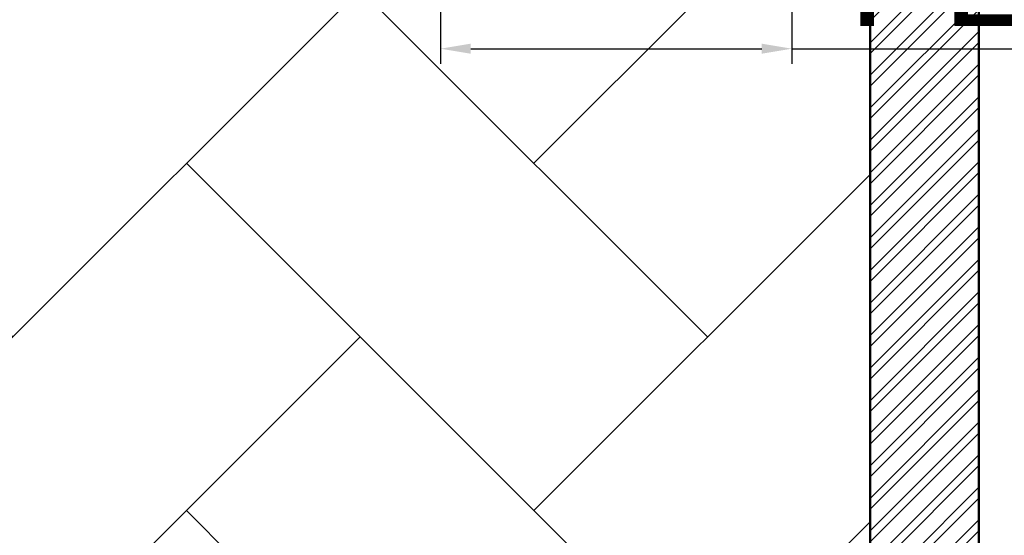
# Model space of a CAD drawing. Units: inches. Extents: x 3590 to 5167, y 65 to 1917.
# Tile 70 of 100: x 5001 to 5082, y 1722 to 1765. Entities that reach past the tile are written whole.
import ezdxf

# ---------------------------------------------------------------- set-up
doc = ezdxf.new("R2010")
doc.units = ezdxf.units.IN
for name, color, linetype, lineweight in [('A-ANNO-DIMS', 2, 'Continuous', 18), ('A-FLOR-PATT', 8, 'Continuous', 13), ('A-WALL', 7, 'Continuous', 50), ('A-WALL-PATT', 251, 'Continuous', 13)]:
    doc.layers.add(name, color=color, linetype=linetype, lineweight=lineweight)
doc.styles.get("Standard").update_dxf_attribs({"font": 'arial.ttf'})
doc.dimstyles.new('ISO-25', dxfattribs={"dimtxt": 9, "dimasz": 2.5, "dimexe": 1.25, "dimexo": 0.625, "dimtad": 1, "dimdec": 1, "dimlunit": 3, "dimtxsty": 'Standard', "dimcen": 2.5, "dimadec": 0, "dimazin": 0, "dimtfac": 1, "dimtdec": 1, "dimtmove": 0, "dimatfit": 3, "dimfxl": 1, "dimarcsym": 0})

# ---------------------------------------------------------------- blocks, each defined once
blk = doc.blocks.new('*D322')
at = {"layer": 'A-ANNO-DIMS', "color": 0, "lineweight": -2, "transparency": 16777216}
for p, q in [((5035.744, 1766.184), (5035.744, 1761.199)), ((5064.812, 1766.184), (5064.812, 1761.199)), ((5038.244, 1762.449), (5062.312, 1762.449)), ((5064.812, 1762.449), (5166.991, 1762.449))]:
    blk.add_line(p, q, dxfattribs=at)
at = {"layer": 'A-ANNO-DIMS', "color": 0, "transparency": 16777216}
for points in [[(5038.244, 1762.866), (5038.244, 1762.032), (5035.744, 1762.449)], [(5062.312, 1762.866), (5062.312, 1762.032), (5064.812, 1762.449)]]:
    blk.add_solid(points, dxfattribs=at)
at = {"layer": 'Defpoints', "color": 0, "transparency": 16777216}
for p in [(5035.744, 1766.809), (5064.812, 1766.809), (5064.812, 1762.449)]:
    blk.add_point(p, dxfattribs=at)
at = {"layer": 'A-ANNO-DIMS', "color": 0, "transparency": 16777216, "insert": (5117.152, 1767.669), "char_height": 9, "attachment_point": 5}
blk.add_mtext('PLANT 2\'-5" TYP.', dxfattribs=at)

msp = doc.modelspace()

# ---------------------------------------------------------------- hatches: boundary and pattern name
at = {"layer": 'A-FLOR-PATT', "transparency": 33554687}
h = msp.add_hatch(dxfattribs=at)
h.set_pattern_fill('AR-HBONE', color=256, scale=0.2)
h.set_pattern_definition([(45, (-588.972, 0), (0, 28.73682), [60.96, -20.32]), (135, (-574.604, 14.368), (3e-15, 28.73682), [60.96, -20.32])])
h.paths.add_polyline_path([(5071.274, 1796.999), (4933.274, 1796.999), (4933.274, 1753.999), (4962.774, 1753.999, -0.414214), (4928.774, 1719.999), (4933.274, 1718.999), (4933.274, 1334.999), (5071.274, 1334.999)])
h.paths.add_polyline_path([(4951.78, 1521.077), (4951.715, 1521.04), (4951.563, 1520.895)], flags=16)
h.paths.add_polyline_path([(4952.267, 1521.376), (4952.198, 1521.371), (4952.198, 1521.356)], flags=0)
h.paths.add_polyline_path([(4967.051, 1529.728), (4965.231, 1528.694), (4963.411, 1527.714), (4961.756, 1526.851), (4963.589, 1527.449), (4964.036, 1527.478), (4962.975, 1527.249), (4961.76, 1526.852), (4959.792, 1525.834), (4958.005, 1524.895), (4956.24, 1523.93), (4954.504, 1522.919), (4954.129, 1522.682), (4953.361, 1521.997), (4953.366, 1521.998), (4953.605, 1522.064), (4955.106, 1522.761), (4956.921, 1523.434), (4958.678, 1523.915), (4960.358, 1524.2), (4961.945, 1524.286), (4964.171, 1524.108), (4965.958, 1523.309), (4963.863, 1522.976), (4965.187, 1522.499), (4963.366, 1522.497), (4961.545, 1522.487), (4959.764, 1522.461), (4958.304, 1522.419), (4957.974, 1522.388), (4956.307, 1522.232), (4954.718, 1522.071), (4953.251, 1521.899), (4953.525, 1521.623), (4954.331, 1521.379), (4956.243, 1521.23), (4958.039, 1520.93), (4959.684, 1520.483), (4961.16, 1519.896), (4963.107, 1518.8), (4964.393, 1517.325), (4962.973, 1517.726), (4964.558, 1516.661), (4965.407, 1515.708), (4963.507, 1516.322), (4961.68, 1517.005), (4959.935, 1517.745), (4958.282, 1518.528), (4956.732, 1519.343), (4955.295, 1520.175), (4954.672, 1520.572), (4954.513, 1520.627), (4955.658, 1519.318), (4956.703, 1517.982), (4957.644, 1516.647), (4958.485, 1515.334), (4959.55, 1513.524), (4960.438, 1511.769), (4958.841, 1513.62), (4957.452, 1515.325), (4955.819, 1517.459), (4956.665, 1515.448), (4957.111, 1513.923), (4957.447, 1511.714), (4957.076, 1509.793), (4956.538, 1511.11), (4955.992, 1512.569), (4955.444, 1514.125), (4954.898, 1515.735), (4954.357, 1517.356), (4953.824, 1518.943), (4953.305, 1520.452), (4953.065, 1521.116), (4952.971, 1521.146), (4952.949, 1521.086), (4952.73, 1520.199), (4953.37, 1518.024), (4953.757, 1516.373), (4954.051, 1514.765), (4954.264, 1513.221), (4954.471, 1511.131), (4954.497, 1510.402), (4954.409, 1511.76), (4954.264, 1513.221), (4954.051, 1514.765), (4953.757, 1516.373), (4953.37, 1518.024), (4952.877, 1519.698), (4952.716, 1520.141), (4952.533, 1519.059), (4952.374, 1517.789), (4952.219, 1516.312), (4952.046, 1514.6), (4951.833, 1512.626), (4951.557, 1510.363), (4951.203, 1512.168), (4950.852, 1514.339), (4950.985, 1516.376), (4951.66, 1518.286), (4952.593, 1520.481), (4952.357, 1521.13), (4951.855, 1520.328), (4950.839, 1518.908), (4949.777, 1517.587), (4948.916, 1516.617), (4948.111, 1515.256), (4947.089, 1513.554), (4945.889, 1511.615), (4946.326, 1513.402), (4946.562, 1514.249), (4945.528, 1513.327), (4944.581, 1512.531), (4946.018, 1514.508), (4947.204, 1516.048), (4947.893, 1517.313), (4949.307, 1518.764), (4950.414, 1519.767), (4950.451, 1519.806), (4952.267, 1521.376), (4951.645, 1521.493), (4950.404, 1521.18), (4948.044, 1520.359), (4946.119, 1519.452), (4944.572, 1518.475), (4943.35, 1517.443), (4941.997, 1515.92), (4941.661, 1515.275), (4942.813, 1516.99), (4944.572, 1518.475), (4946.119, 1519.452), (4948.044, 1520.359), (4950.404, 1521.18), (4951.645, 1521.493), (4949.647, 1521.868), (4948.6, 1521.756), (4947.126, 1521.57), (4945.42, 1521.348), (4943.45, 1521.105), (4941.183, 1520.856), (4942.86, 1521.613), (4943.873, 1522.03), (4942.952, 1521.909), (4941.41, 1521.485), (4939.543, 1520.67), (4938.968, 1520.226), (4940.733, 1521.299), (4942.952, 1521.909), (4943.702, 1522.008), (4945.894, 1522.7), (4947.565, 1522.714), (4948.921, 1522.566), (4951.131, 1522.183), (4950.971, 1522.297), (4948.129, 1523.006), (4946.035, 1523.707), (4944.232, 1524.521), (4942.707, 1525.461), (4941.444, 1526.537), (4940.43, 1527.761), (4939.649, 1529.143), (4941.421, 1528.122), (4943.147, 1527.132), (4944.841, 1526.175), (4946.514, 1525.25), (4948.179, 1524.359), (4948.365, 1524.263), (4946.475, 1526.045), (4945.181, 1527.54), (4944.19, 1529.033), (4943.496, 1530.54), (4943.278, 1531.36), (4942.498, 1531.919), (4943.114, 1531.762), (4942.959, 1533.659), (4944.14, 1531.989), (4944.612, 1531.323), (4946.202, 1530.463), (4947.486, 1529.509), (4948.79, 1528.226), (4950.368, 1526.237), (4949.485, 1528.155), (4948.851, 1530.123), (4948.491, 1532.041), (4948.381, 1533.918), (4948.501, 1535.76), (4948.827, 1537.573), (4949.418, 1535.565), (4949.957, 1533.569), (4950.464, 1531.586), (4950.961, 1529.617), (4951.391, 1527.954), (4951.724, 1530.687), (4952.201, 1532.58), (4952.889, 1534.33), (4953.77, 1535.951), (4954.827, 1537.46), (4954.521, 1535.39), (4954.273, 1533.937), (4955.58, 1535.663), (4956.748, 1536.739), (4956.159, 1534.78), (4955.589, 1532.873), (4955.043, 1531.006), (4954.525, 1529.166), (4954.038, 1527.341), (4953.638, 1525.733), (4953.611, 1525.586), (4953.398, 1524.166), (4953.382, 1524.009), (4954.07, 1525.476), (4954.912, 1527.022), (4956.136, 1528.894), (4957.847, 1530.577), (4959.376, 1531.54), (4958.256, 1530.104), (4957.143, 1528.663), (4956.066, 1527.243), (4955.056, 1525.871), (4954.141, 1524.571), (4953.352, 1523.372), (4953.311, 1523.303), (4953.273, 1522.925), (4953.261, 1522.382), (4954.103, 1523.373), (4954.63, 1524.284), (4955.961, 1526.358), (4957.23, 1528.13), (4958.421, 1529.609), (4960.037, 1531.368), (4961.374, 1532.375), (4962.101, 1532.77), (4961.07, 1531.061), (4959.987, 1529.438), (4958.869, 1527.908), (4958.15, 1527.007), (4959.803, 1528.003), (4961.589, 1528.793), (4963.391, 1529.328), (4965.211, 1529.632)], flags=16)
h.paths.add_polyline_path([(4962.944, 1523.182), (4961.107, 1523.422), (4960.392, 1523.362), (4962.35, 1523.331)], flags=0)
h.paths.add_polyline_path([(5049.541, 1584.551), (5049.476, 1584.515), (5049.325, 1584.37)], flags=16)
h.paths.add_polyline_path([(5050.028, 1584.851), (5049.959, 1584.845), (5049.959, 1584.83)], flags=0)
h.paths.add_polyline_path([(5042.333, 1581.949), (5043.88, 1582.926), (5045.806, 1583.833), (5048.165, 1584.654), (5049.406, 1584.967), (5047.408, 1585.342), (5046.361, 1585.231), (5044.888, 1585.044), (5043.181, 1584.822), (5041.211, 1584.579), (5038.944, 1584.33), (5040.622, 1585.087), (5041.634, 1585.504), (5040.713, 1585.383), (5039.171, 1584.959), (5037.304, 1584.144), (5036.729, 1583.7), (5038.494, 1584.773), (5040.713, 1585.383), (5041.463, 1585.482), (5043.655, 1586.174), (5045.326, 1586.188), (5046.682, 1586.04), (5048.893, 1585.657), (5048.732, 1585.771), (5045.891, 1586.48), (5043.796, 1587.181), (5041.994, 1587.996), (5040.468, 1588.935), (5039.205, 1590.011), (5038.191, 1591.235), (5037.41, 1592.617), (5039.182, 1591.596), (5040.909, 1590.607), (5042.602, 1589.649), (5044.275, 1588.724), (5045.94, 1587.833), (5046.126, 1587.738), (5044.237, 1589.519), (5042.942, 1591.015), (5041.952, 1592.508), (5041.257, 1594.014), (5041.039, 1594.834), (5040.26, 1595.393), (5040.875, 1595.237), (5040.721, 1597.133), (5041.901, 1595.463), (5042.373, 1594.798), (5043.963, 1593.938), (5045.247, 1592.983), (5046.552, 1591.701), (5048.129, 1589.712), (5047.247, 1591.63), (5046.613, 1593.597), (5046.252, 1595.515), (5046.142, 1597.392), (5046.262, 1599.234), (5046.588, 1601.047), (5047.179, 1599.039), (5047.718, 1597.043), (5048.225, 1595.06), (5048.722, 1593.091), (5049.152, 1591.429), (5049.485, 1594.161), (5049.962, 1596.054), (5050.65, 1597.804), (5051.532, 1599.425), (5052.589, 1600.934), (5052.283, 1598.864), (5052.034, 1597.411), (5053.341, 1599.137), (5054.509, 1600.213), (5053.92, 1598.254), (5053.35, 1596.348), (5052.805, 1594.48), (5052.286, 1592.64), (5051.799, 1590.815), (5051.4, 1589.207), (5051.373, 1589.06), (5051.159, 1587.64), (5051.143, 1587.483), (5051.831, 1588.95), (5052.673, 1590.496), (5053.898, 1592.368), (5055.608, 1594.051), (5057.137, 1595.014), (5056.017, 1593.578), (5054.904, 1592.137), (5053.828, 1590.717), (5052.817, 1589.345), (5051.902, 1588.046), (5051.113, 1586.846), (5051.072, 1586.777), (5051.034, 1586.399), (5051.022, 1585.856), (5051.864, 1586.847), (5052.391, 1587.758), (5053.723, 1589.832), (5054.991, 1591.604), (5056.182, 1593.083), (5057.798, 1594.842), (5059.135, 1595.849), (5059.863, 1596.244), (5058.831, 1594.535), (5057.749, 1592.912), (5056.63, 1591.382), (5055.912, 1590.482), (5057.564, 1591.477), (5059.35, 1592.267), (5061.152, 1592.802), (5062.972, 1593.106), (5064.812, 1593.203), (5062.992, 1592.169), (5061.172, 1591.188), (5059.518, 1590.325), (5061.35, 1590.924), (5061.797, 1590.952), (5060.737, 1590.723), (5059.521, 1590.326), (5057.553, 1589.308), (5055.766, 1588.369), (5054.002, 1587.404), (5052.265, 1586.393), (5051.891, 1586.156), (5051.122, 1585.471), (5051.127, 1585.472), (5051.366, 1585.538), (5052.867, 1586.235), (5054.682, 1586.908), (5056.439, 1587.389), (5058.12, 1587.675), (5059.706, 1587.76), (5061.933, 1587.583), (5063.719, 1586.783), (5061.624, 1586.45), (5062.949, 1585.973), (5061.127, 1585.971), (5059.307, 1585.961), (5057.525, 1585.935), (5056.065, 1585.893), (5055.735, 1585.862), (5054.068, 1585.707), (5052.479, 1585.546), (5051.012, 1585.373), (5051.286, 1585.097), (5052.092, 1584.853), (5054.004, 1584.704), (5055.8, 1584.404), (5057.446, 1583.958), (5058.921, 1583.37), (5060.868, 1582.274), (5062.154, 1580.799), (5060.734, 1581.2), (5062.32, 1580.135), (5063.168, 1579.182), (5061.269, 1579.796), (5059.441, 1580.479), (5057.696, 1581.219), (5056.043, 1582.003), (5054.493, 1582.817), (5053.057, 1583.649), (5052.433, 1584.047), (5052.274, 1584.101), (5053.42, 1582.793), (5054.464, 1581.457), (5055.405, 1580.121), (5056.247, 1578.809), (5057.311, 1576.998), (5058.199, 1575.244), (5056.602, 1577.094), (5055.213, 1578.799), (5053.58, 1580.933), (5054.427, 1578.922), (5054.872, 1577.397), (5055.208, 1575.189), (5054.838, 1573.267), (5054.299, 1574.584), (5053.754, 1576.043), (5053.206, 1577.599), (5052.659, 1579.209), (5052.118, 1580.83), (5051.585, 1582.417), (5051.066, 1583.927), (5050.826, 1584.59), (5050.733, 1584.62), (5050.711, 1584.561), (5050.491, 1583.673), (5051.131, 1581.498), (5051.518, 1579.847), (5051.813, 1578.24), (5052.026, 1576.695), (5052.233, 1574.605), (5052.258, 1573.876), (5052.17, 1575.234), (5052.026, 1576.695), (5051.813, 1578.24), (5051.518, 1579.847), (5051.131, 1581.498), (5050.638, 1583.172), (5050.477, 1583.615), (5050.294, 1582.533), (5050.136, 1581.263), (5049.981, 1579.786), (5049.807, 1578.074), (5049.594, 1576.1), (5049.318, 1573.837), (5048.965, 1575.642), (5048.613, 1577.813), (5048.747, 1579.85), (5049.421, 1581.76), (5050.354, 1583.955), (5050.118, 1584.604), (5049.616, 1583.802), (5048.6, 1582.382), (5047.538, 1581.061), (5046.677, 1580.091), (5045.872, 1578.73), (5044.85, 1577.028), (5043.651, 1575.089), (5044.087, 1576.877), (5044.324, 1577.723), (5043.289, 1576.801), (5042.342, 1576.005), (5043.779, 1577.982), (5044.966, 1579.522), (5045.655, 1580.787), (5047.068, 1582.239), (5048.175, 1583.241), (5048.213, 1583.28), (5050.028, 1584.851), (5049.406, 1584.967), (5048.165, 1584.654), (5045.806, 1583.833), (5043.88, 1582.926), (5042.333, 1581.949), (5041.111, 1580.917), (5039.758, 1579.394), (5039.423, 1578.749), (5040.575, 1580.464)], flags=16)
h.paths.add_polyline_path([(4954.799, 1533.12), (4954.262, 1532.079), (4953.831, 1530.935), (4953.505, 1529.636), (4953.283, 1528.133), (4953.167, 1526.376), (4953.156, 1524.315), (4953.277, 1521.236), (4952.802, 1521.842), (4951.557, 1521.998), (4950.976, 1521.961), (4952.661, 1521.941), (4952.802, 1521.842), (4953.152, 1523.593), (4953.167, 1526.376), (4953.283, 1528.133), (4953.609, 1530.346), (4954.456, 1532.592)], flags=0)
h.paths.add_polyline_path([(5050.563, 1585.316), (5049.318, 1585.472), (5048.737, 1585.435), (5050.422, 1585.415), (5050.563, 1585.316), (5050.914, 1587.067), (5050.928, 1589.851), (5051.045, 1591.607), (5051.371, 1593.82), (5052.217, 1596.066), (5052.56, 1596.594), (5052.024, 1595.554), (5051.592, 1594.409), (5051.266, 1593.11), (5051.045, 1591.607), (5050.928, 1589.851), (5050.918, 1587.789), (5051.038, 1584.71)], flags=0)
h.paths.add_polyline_path([(5058.153, 1586.836), (5060.111, 1586.805), (5060.705, 1586.656), (5058.868, 1586.896)], flags=0)
h.paths.add_polyline_path([(5049.541, 1430.936), (5049.476, 1430.9), (5049.325, 1430.755)], flags=16)
h.paths.add_polyline_path([(5050.028, 1431.236), (5049.959, 1431.231), (5049.959, 1431.215)], flags=0)
h.paths.add_polyline_path([(5046.588, 1447.432), (5047.179, 1445.425), (5047.718, 1443.429), (5048.225, 1441.446), (5048.722, 1439.476), (5049.152, 1437.814), (5049.485, 1440.546), (5049.962, 1442.439), (5050.65, 1444.189), (5051.532, 1445.811), (5052.589, 1447.319), (5052.283, 1445.249), (5052.034, 1443.796), (5053.341, 1445.522), (5054.509, 1446.598), (5053.92, 1444.64), (5053.35, 1442.733), (5052.805, 1440.865), (5052.286, 1439.025), (5051.799, 1437.201), (5051.4, 1435.592), (5051.373, 1435.445), (5051.159, 1434.025), (5051.143, 1433.868), (5051.831, 1435.335), (5052.673, 1436.881), (5053.898, 1438.753), (5055.608, 1440.436), (5057.137, 1441.4), (5056.017, 1439.963), (5054.904, 1438.522), (5053.828, 1437.102), (5052.817, 1435.73), (5051.902, 1434.431), (5051.113, 1433.231), (5051.072, 1433.162), (5051.034, 1432.784), (5051.022, 1432.242), (5051.864, 1433.232), (5052.391, 1434.143), (5053.723, 1436.217), (5054.991, 1437.989), (5056.182, 1439.468), (5057.798, 1441.227), (5059.135, 1442.235), (5059.863, 1442.629), (5058.831, 1440.921), (5057.749, 1439.298), (5056.63, 1437.767), (5055.912, 1436.867), (5057.564, 1437.863), (5059.35, 1438.652), (5061.152, 1439.187), (5062.972, 1439.491), (5064.812, 1439.588), (5062.992, 1438.554), (5061.172, 1437.573), (5059.518, 1436.71), (5061.35, 1437.309), (5061.797, 1437.337), (5060.737, 1437.108), (5059.521, 1436.711), (5057.553, 1435.693), (5055.766, 1434.754), (5054.002, 1433.789), (5052.265, 1432.778), (5051.891, 1432.541), (5051.122, 1431.856), (5051.127, 1431.857), (5051.366, 1431.923), (5052.867, 1432.62), (5054.682, 1433.293), (5056.439, 1433.775), (5058.12, 1434.06), (5059.706, 1434.145), (5061.933, 1433.968), (5063.719, 1433.168), (5061.624, 1432.835), (5062.949, 1432.358), (5061.127, 1432.357), (5059.307, 1432.346), (5057.525, 1432.32), (5056.065, 1432.278), (5055.735, 1432.248), (5054.068, 1432.092), (5052.479, 1431.931), (5051.012, 1431.759), (5051.286, 1431.482), (5052.092, 1431.238), (5054.004, 1431.089), (5055.8, 1430.789), (5057.446, 1430.343), (5058.921, 1429.755), (5060.868, 1428.66), (5062.154, 1427.185), (5060.734, 1427.585), (5062.32, 1426.52), (5063.168, 1425.567), (5061.269, 1426.181), (5059.441, 1426.865), (5057.696, 1427.604), (5056.043, 1428.388), (5054.493, 1429.202), (5053.057, 1430.034), (5052.433, 1430.432), (5052.274, 1430.487), (5053.42, 1429.178), (5054.464, 1427.842), (5055.405, 1426.506), (5056.247, 1425.194), (5057.311, 1423.383), (5058.199, 1421.629), (5056.602, 1423.479), (5055.213, 1425.184), (5053.58, 1427.318), (5054.427, 1425.307), (5054.872, 1423.782), (5055.208, 1421.574), (5054.838, 1419.652), (5054.299, 1420.97), (5053.754, 1422.428), (5053.206, 1423.984), (5052.659, 1425.595), (5052.118, 1427.215), (5051.585, 1428.802), (5051.066, 1430.312), (5050.826, 1430.975), (5050.733, 1431.005), (5050.711, 1430.946), (5050.491, 1430.058), (5051.131, 1427.883), (5051.518, 1426.232), (5051.813, 1424.625), (5052.026, 1423.081), (5052.233, 1420.991), (5052.258, 1420.261), (5052.17, 1421.619), (5052.026, 1423.081), (5051.813, 1424.625), (5051.518, 1426.232), (5051.131, 1427.883), (5050.638, 1429.558), (5050.477, 1430.001), (5050.294, 1428.918), (5050.136, 1427.648), (5049.981, 1426.171), (5049.807, 1424.459), (5049.594, 1422.485), (5049.318, 1420.222), (5048.965, 1422.028), (5048.613, 1424.199), (5048.747, 1426.235), (5049.421, 1428.146), (5050.354, 1430.34), (5050.118, 1430.989), (5049.616, 1430.187), (5048.6, 1428.768), (5047.538, 1427.446), (5046.677, 1426.477), (5045.872, 1425.116), (5044.85, 1423.413), (5043.651, 1421.474), (5044.087, 1423.262), (5044.324, 1424.109), (5043.289, 1423.186), (5042.342, 1422.391), (5043.779, 1424.368), (5044.966, 1425.907), (5045.655, 1427.173), (5047.068, 1428.624), (5048.175, 1429.627), (5048.213, 1429.666), (5050.028, 1431.236), (5049.406, 1431.353), (5048.165, 1431.039), (5045.806, 1430.218), (5043.88, 1429.311), (5042.333, 1428.334), (5041.111, 1427.302), (5039.758, 1425.779), (5039.423, 1425.134), (5040.575, 1426.849), (5042.333, 1428.334), (5043.88, 1429.311), (5045.806, 1430.218), (5048.165, 1431.039), (5049.406, 1431.353), (5047.408, 1431.727), (5046.361, 1431.616), (5044.888, 1431.429), (5043.181, 1431.207), (5041.211, 1430.964), (5038.944, 1430.715), (5040.622, 1431.472), (5041.634, 1431.89), (5040.713, 1431.769), (5039.171, 1431.345), (5037.304, 1430.53), (5036.729, 1430.085), (5038.494, 1431.158), (5040.713, 1431.769), (5041.463, 1431.867), (5043.655, 1432.559), (5045.326, 1432.573), (5046.682, 1432.425), (5048.893, 1432.042), (5048.732, 1432.156), (5045.891, 1432.865), (5043.796, 1433.566), (5041.994, 1434.381), (5040.468, 1435.321), (5039.205, 1436.396), (5038.191, 1437.62), (5037.41, 1439.002), (5039.182, 1437.982), (5040.909, 1436.992), (5042.602, 1436.034), (5044.275, 1435.109), (5045.94, 1434.218), (5046.126, 1434.123), (5044.237, 1435.904), (5042.942, 1437.4), (5041.952, 1438.893), (5041.257, 1440.399), (5041.039, 1441.219), (5040.26, 1441.778), (5040.875, 1441.622), (5040.721, 1443.518), (5041.901, 1441.848), (5042.373, 1441.183), (5043.963, 1440.323), (5045.247, 1439.369), (5046.552, 1438.086), (5048.129, 1436.097), (5047.247, 1438.015), (5046.613, 1439.982), (5046.252, 1441.901), (5046.142, 1443.778), (5046.262, 1445.619)], flags=16)
h.paths.add_polyline_path([(5052.382, 1444.255), (5051.623, 1442.78), (5052.024, 1441.939), (5052.56, 1442.98)], flags=0)
h.paths.add_polyline_path([(5050.563, 1431.701), (5049.318, 1431.857), (5048.737, 1431.821), (5050.422, 1431.8)], flags=0)
h.paths.add_polyline_path([(5058.153, 1433.221), (5060.111, 1433.19), (5060.705, 1433.041), (5058.868, 1433.281)], flags=0)
h.paths.add_polyline_path([(5049.541, 1352.285), (5049.476, 1352.249), (5049.325, 1352.104)], flags=16)
h.paths.add_polyline_path([(5050.028, 1352.585), (5049.959, 1352.58), (5049.959, 1352.564)], flags=0)
h.paths.add_polyline_path([(5046.588, 1368.781), (5047.179, 1366.774), (5047.718, 1364.778), (5048.225, 1362.795), (5048.722, 1360.825), (5049.152, 1359.163), (5049.485, 1361.896), (5049.962, 1363.789), (5050.65, 1365.538), (5051.532, 1367.16), (5052.589, 1368.669), (5052.283, 1366.598), (5052.034, 1365.145), (5053.341, 1366.871), (5054.509, 1367.947), (5053.92, 1365.989), (5053.35, 1364.082), (5052.805, 1362.214), (5052.286, 1360.374), (5051.799, 1358.55), (5051.4, 1356.942), (5051.373, 1356.794), (5051.159, 1355.374), (5051.143, 1355.218), (5051.831, 1356.684), (5052.673, 1358.23), (5053.898, 1360.102), (5055.608, 1361.786), (5057.137, 1362.749), (5056.017, 1361.313), (5054.904, 1359.872), (5053.828, 1358.452), (5052.817, 1357.079), (5051.902, 1355.78), (5051.113, 1354.581), (5051.072, 1354.512), (5051.034, 1354.133), (5051.022, 1353.591), (5051.864, 1354.581), (5052.391, 1355.492), (5053.723, 1357.566), (5054.991, 1359.338), (5056.182, 1360.817), (5057.798, 1362.577), (5059.135, 1363.584), (5059.863, 1363.979), (5058.831, 1362.27), (5057.749, 1360.647), (5056.63, 1359.117), (5055.912, 1358.216), (5057.564, 1359.212), (5059.35, 1360.001), (5061.152, 1360.536), (5062.972, 1360.841), (5064.812, 1360.937), (5062.992, 1359.903), (5061.172, 1358.923), (5059.518, 1358.059), (5061.35, 1358.658), (5061.797, 1358.687), (5060.737, 1358.458), (5059.521, 1358.061), (5057.553, 1357.043), (5055.766, 1356.103), (5054.002, 1355.138), (5052.265, 1354.127), (5051.891, 1353.89), (5051.122, 1353.206), (5051.127, 1353.206), (5051.366, 1353.272), (5052.867, 1353.969), (5054.682, 1354.643), (5056.439, 1355.124), (5058.12, 1355.409), (5059.706, 1355.495), (5061.933, 1355.317), (5063.719, 1354.518), (5061.624, 1354.184), (5062.949, 1353.708), (5061.127, 1353.706), (5059.307, 1353.695), (5057.525, 1353.669), (5056.065, 1353.627), (5055.735, 1353.597), (5054.068, 1353.441), (5052.479, 1353.28), (5051.012, 1353.108), (5051.286, 1352.831), (5052.092, 1352.587), (5054.004, 1352.439), (5055.8, 1352.138), (5057.446, 1351.692), (5058.921, 1351.104), (5060.868, 1350.009), (5062.154, 1348.534), (5060.734, 1348.935), (5062.32, 1347.869), (5063.168, 1346.916), (5061.269, 1347.53), (5059.441, 1348.214), (5057.696, 1348.954), (5056.043, 1349.737), (5054.493, 1350.551), (5053.057, 1351.383), (5052.433, 1351.781), (5052.274, 1351.836), (5053.42, 1350.527), (5054.464, 1349.191), (5055.405, 1347.855), (5056.247, 1346.543), (5057.311, 1344.733), (5058.199, 1342.978), (5056.602, 1344.828), (5055.213, 1346.534), (5053.58, 1348.667), (5054.427, 1346.656), (5054.872, 1345.132), (5055.208, 1342.923), (5054.838, 1341.002), (5054.299, 1342.319), (5053.754, 1343.778), (5053.206, 1345.334), (5052.659, 1346.944), (5052.118, 1348.564), (5051.585, 1350.151), (5051.066, 1351.661), (5050.826, 1352.324), (5050.733, 1352.355), (5050.711, 1352.295), (5050.491, 1351.408), (5051.131, 1349.232), (5051.518, 1347.581), (5051.813, 1345.974), (5052.026, 1344.43), (5052.233, 1342.34), (5052.258, 1341.61), (5052.17, 1342.969), (5052.026, 1344.43), (5051.813, 1345.974), (5051.518, 1347.581), (5051.131, 1349.232), (5050.638, 1350.907), (5050.477, 1351.35), (5050.294, 1350.267), (5050.136, 1348.997), (5049.981, 1347.52), (5049.807, 1345.809), (5049.594, 1343.835), (5049.318, 1341.571), (5048.965, 1343.377), (5048.613, 1345.548), (5048.747, 1347.585), (5049.421, 1349.495), (5050.354, 1351.689), (5050.118, 1352.339), (5049.616, 1351.536), (5048.6, 1350.117), (5047.538, 1348.795), (5046.677, 1347.826), (5045.872, 1346.465), (5044.85, 1344.763), (5043.651, 1342.824), (5044.087, 1344.611), (5044.324, 1345.458), (5043.289, 1344.535), (5042.342, 1343.74), (5043.779, 1345.717), (5044.966, 1347.256), (5045.655, 1348.522), (5047.068, 1349.973), (5048.175, 1350.976), (5048.213, 1351.015), (5050.028, 1352.585), (5049.406, 1352.702), (5048.165, 1352.388), (5045.806, 1351.567), (5043.88, 1350.661), (5042.333, 1349.683), (5041.111, 1348.651), (5039.758, 1347.128), (5039.423, 1346.483), (5040.575, 1348.198), (5042.333, 1349.683), (5043.88, 1350.661), (5045.806, 1351.567), (5048.165, 1352.388), (5049.406, 1352.702), (5047.408, 1353.076), (5046.361, 1352.965), (5044.888, 1352.779), (5043.181, 1352.556), (5041.211, 1352.313), (5038.944, 1352.065), (5040.622, 1352.821), (5041.634, 1353.239), (5040.713, 1353.118), (5039.171, 1352.694), (5037.304, 1351.879), (5036.729, 1351.434), (5038.494, 1352.508), (5040.713, 1353.118), (5041.463, 1353.216), (5043.655, 1353.909), (5045.326, 1353.923), (5046.682, 1353.774), (5048.893, 1353.391), (5048.732, 1353.506), (5045.891, 1354.214), (5043.796, 1354.915), (5041.994, 1355.73), (5040.468, 1356.67), (5039.205, 1357.746), (5038.191, 1358.969), (5037.41, 1360.352), (5039.182, 1359.331), (5040.909, 1358.341), (5042.602, 1357.383), (5044.275, 1356.458), (5045.94, 1355.567), (5046.126, 1355.472), (5044.237, 1357.253), (5042.942, 1358.749), (5041.952, 1360.242), (5041.257, 1361.748), (5041.039, 1362.568), (5040.26, 1363.128), (5040.875, 1362.971), (5040.721, 1364.867), (5041.901, 1363.197), (5042.373, 1362.532), (5043.963, 1361.672), (5045.247, 1360.718), (5046.552, 1359.435), (5048.129, 1357.446), (5047.247, 1359.364), (5046.613, 1361.331), (5046.252, 1363.25), (5046.142, 1365.127), (5046.262, 1366.969)], flags=16)
h.paths.add_polyline_path([(5052.382, 1365.604), (5051.623, 1364.129), (5052.024, 1363.288), (5052.56, 1364.329)], flags=0)
h.paths.add_polyline_path([(4951.78, 1698.041), (4951.715, 1698.005), (4951.563, 1697.859)], flags=16)
h.paths.add_polyline_path([(4952.267, 1698.341), (4952.198, 1698.335), (4952.198, 1698.32)], flags=0)
h.paths.add_polyline_path([(4957.076, 1686.757), (4956.538, 1688.074), (4955.992, 1689.533), (4955.444, 1691.089), (4954.898, 1692.699), (4954.357, 1694.32), (4953.824, 1695.907), (4953.305, 1697.417), (4953.065, 1698.08), (4952.971, 1698.11), (4952.949, 1698.051), (4952.73, 1697.163), (4953.37, 1694.988), (4953.757, 1693.337), (4954.051, 1691.729), (4954.264, 1690.185), (4954.471, 1688.095), (4954.497, 1687.366), (4954.409, 1688.724), (4954.264, 1690.185), (4954.051, 1691.729), (4953.757, 1693.337), (4953.37, 1694.988), (4952.877, 1696.662), (4952.716, 1697.105), (4952.533, 1696.023), (4952.374, 1694.753), (4952.219, 1693.276), (4952.046, 1691.564), (4951.833, 1689.59), (4951.557, 1687.327), (4951.203, 1689.132), (4950.852, 1691.303), (4950.985, 1693.34), (4951.66, 1695.25), (4952.593, 1697.445), (4952.357, 1698.094), (4951.855, 1697.292), (4950.839, 1695.872), (4949.777, 1694.551), (4948.916, 1693.581), (4948.111, 1692.22), (4947.089, 1690.518), (4945.889, 1688.579), (4946.326, 1690.366), (4946.562, 1691.213), (4945.528, 1690.291), (4944.581, 1689.495), (4946.018, 1691.472), (4947.204, 1693.012), (4947.893, 1694.277), (4949.307, 1695.729), (4950.414, 1696.731), (4950.451, 1696.77), (4952.267, 1698.341), (4951.645, 1698.457), (4950.404, 1698.144), (4948.044, 1697.323), (4946.119, 1696.416), (4944.572, 1695.439), (4943.35, 1694.407), (4941.997, 1692.884), (4941.661, 1692.239), (4942.813, 1693.954), (4944.572, 1695.439), (4946.119, 1696.416), (4948.044, 1697.323), (4950.404, 1698.144), (4951.645, 1698.457), (4949.647, 1698.832), (4948.6, 1698.72), (4947.126, 1698.534), (4945.42, 1698.312), (4943.45, 1698.069), (4941.183, 1697.82), (4942.86, 1698.577), (4943.873, 1698.994), (4942.952, 1698.873), (4941.41, 1698.449), (4939.543, 1697.634), (4938.968, 1697.19), (4940.733, 1698.263), (4942.952, 1698.873), (4943.702, 1698.972), (4945.894, 1699.664), (4947.565, 1699.678), (4948.921, 1699.53), (4951.131, 1699.147), (4950.971, 1699.261), (4948.129, 1699.97), (4946.035, 1700.671), (4944.232, 1701.486), (4942.707, 1702.425), (4941.444, 1703.501), (4940.43, 1704.725), (4939.649, 1706.107), (4941.421, 1705.086), (4943.147, 1704.097), (4944.841, 1703.139), (4946.514, 1702.214), (4948.179, 1701.323), (4948.365, 1701.227), (4946.475, 1703.009), (4945.181, 1704.505), (4944.19, 1705.997), (4943.496, 1707.504), (4943.278, 1708.324), (4942.498, 1708.883), (4943.114, 1708.727), (4942.959, 1710.623), (4944.14, 1708.953), (4944.612, 1708.287), (4946.202, 1707.428), (4947.486, 1706.473), (4948.79, 1705.191), (4950.368, 1703.202), (4949.485, 1705.12), (4948.851, 1707.087), (4948.491, 1709.005), (4948.381, 1710.882), (4948.501, 1712.724), (4948.827, 1714.537), (4949.418, 1712.529), (4949.957, 1710.533), (4950.464, 1708.55), (4950.961, 1706.581), (4951.391, 1704.919), (4951.724, 1707.651), (4952.201, 1709.544), (4952.889, 1711.294), (4953.77, 1712.915), (4954.827, 1714.424), (4954.521, 1712.354), (4954.273, 1710.901), (4955.58, 1712.627), (4956.748, 1713.703), (4956.159, 1711.744), (4955.589, 1709.837), (4955.043, 1707.97), (4954.525, 1706.13), (4954.038, 1704.305), (4953.638, 1702.697), (4953.611, 1702.55), (4953.398, 1701.13), (4953.382, 1700.973), (4954.07, 1702.44), (4954.912, 1703.986), (4956.136, 1705.858), (4957.847, 1707.541), (4959.376, 1708.504), (4958.256, 1707.068), (4957.143, 1705.627), (4956.066, 1704.207), (4955.056, 1702.835), (4954.141, 1701.536), (4953.352, 1700.336), (4953.311, 1700.267), (4953.273, 1699.889), (4953.261, 1699.346), (4954.103, 1700.337), (4954.63, 1701.248), (4955.961, 1703.322), (4957.23, 1705.094), (4958.421, 1706.573), (4960.037, 1708.332), (4961.374, 1709.339), (4962.101, 1709.734), (4961.07, 1708.025), (4959.987, 1706.402), (4958.869, 1704.872), (4958.15, 1703.972), (4959.803, 1704.967), (4961.589, 1705.757), (4963.391, 1706.292), (4965.211, 1706.596), (4967.051, 1706.692), (4965.231, 1705.659), (4963.411, 1704.678), (4961.756, 1703.815), (4963.589, 1704.413), (4964.036, 1704.442), (4962.975, 1704.213), (4961.76, 1703.816), (4959.792, 1702.798), (4958.005, 1701.859), (4956.24, 1700.894), (4954.504, 1699.883), (4954.129, 1699.646), (4953.361, 1698.961), (4953.366, 1698.962), (4953.605, 1699.028), (4955.106, 1699.725), (4956.921, 1700.398), (4958.678, 1700.879), (4960.358, 1701.164), (4961.945, 1701.25), (4964.171, 1701.073), (4965.958, 1700.273), (4963.863, 1699.94), (4965.187, 1699.463), (4963.366, 1699.461), (4961.545, 1699.451), (4959.764, 1699.425), (4958.304, 1699.383), (4957.974, 1699.352), (4956.307, 1699.197), (4954.718, 1699.036), (4953.251, 1698.863), (4953.525, 1698.587), (4954.331, 1698.343), (4956.243, 1698.194), (4958.039, 1697.894), (4959.684, 1697.447), (4961.16, 1696.86), (4963.107, 1695.764), (4964.393, 1694.289), (4962.973, 1694.69), (4964.558, 1693.625), (4965.407, 1692.672), (4963.507, 1693.286), (4961.68, 1693.969), (4959.935, 1694.709), (4958.282, 1695.492), (4956.732, 1696.307), (4955.295, 1697.139), (4954.672, 1697.536), (4954.513, 1697.591), (4955.658, 1696.282), (4956.703, 1694.946), (4957.644, 1693.611), (4958.485, 1692.298), (4959.55, 1690.488), (4960.438, 1688.733), (4958.841, 1690.584), (4957.452, 1692.289), (4955.819, 1694.423), (4956.665, 1692.412), (4957.111, 1690.887), (4957.447, 1688.678)], flags=16)
h.paths.add_polyline_path([(5050.563, 1353.05), (5049.318, 1353.207), (5048.737, 1353.17), (5050.422, 1353.15)], flags=0)
h.paths.add_polyline_path([(4951.78, 1351.486), (4951.715, 1351.45), (4951.563, 1351.305)], flags=16)
h.paths.add_polyline_path([(4952.267, 1351.786), (4952.198, 1351.78), (4952.198, 1351.765)], flags=0)
h.paths.add_polyline_path([(4954.827, 1367.869), (4954.521, 1365.799), (4954.273, 1364.346), (4955.58, 1366.072), (4956.748, 1367.148), (4956.159, 1365.19), (4955.589, 1363.283), (4955.043, 1361.415), (4954.525, 1359.575), (4954.038, 1357.751), (4953.638, 1356.142), (4953.611, 1355.995), (4953.398, 1354.575), (4953.382, 1354.418), (4954.07, 1355.885), (4954.912, 1357.431), (4956.136, 1359.303), (4957.847, 1360.986), (4959.376, 1361.95), (4958.256, 1360.513), (4957.143, 1359.072), (4956.066, 1357.652), (4955.056, 1356.28), (4954.141, 1354.981), (4953.352, 1353.781), (4953.311, 1353.712), (4953.273, 1353.334), (4953.261, 1352.792), (4954.103, 1353.782), (4954.63, 1354.693), (4955.961, 1356.767), (4957.23, 1358.539), (4958.421, 1360.018), (4960.037, 1361.777), (4961.374, 1362.785), (4962.101, 1363.179), (4961.07, 1361.471), (4959.987, 1359.848), (4958.869, 1358.317), (4958.15, 1357.417), (4959.803, 1358.413), (4961.589, 1359.202), (4963.391, 1359.737), (4965.211, 1360.041), (4967.051, 1360.138), (4965.231, 1359.104), (4963.411, 1358.123), (4961.756, 1357.26), (4963.589, 1357.859), (4964.036, 1357.887), (4962.975, 1357.658), (4961.76, 1357.261), (4959.792, 1356.243), (4958.005, 1355.304), (4956.24, 1354.339), (4954.504, 1353.328), (4954.129, 1353.091), (4953.361, 1352.406), (4953.366, 1352.407), (4953.605, 1352.473), (4955.106, 1353.17), (4956.921, 1353.843), (4958.678, 1354.325), (4960.358, 1354.61), (4961.945, 1354.695), (4964.171, 1354.518), (4965.958, 1353.718), (4963.863, 1353.385), (4965.187, 1352.908), (4963.366, 1352.907), (4961.545, 1352.896), (4959.764, 1352.87), (4958.304, 1352.828), (4957.974, 1352.798), (4956.307, 1352.642), (4954.718, 1352.481), (4953.251, 1352.309), (4953.525, 1352.032), (4954.331, 1351.788), (4956.243, 1351.639), (4958.039, 1351.339), (4959.684, 1350.893), (4961.16, 1350.305), (4963.107, 1349.21), (4964.393, 1347.735), (4962.973, 1348.135), (4964.558, 1347.07), (4965.407, 1346.117), (4963.507, 1346.731), (4961.68, 1347.414), (4959.935, 1348.154), (4958.282, 1348.938), (4956.732, 1349.752), (4955.295, 1350.584), (4954.672, 1350.982), (4954.513, 1351.036), (4955.658, 1349.728), (4956.703, 1348.392), (4957.644, 1347.056), (4958.485, 1345.744), (4959.55, 1343.933), (4960.438, 1342.179), (4958.841, 1344.029), (4957.452, 1345.734), (4955.819, 1347.868), (4956.665, 1345.857), (4957.111, 1344.332), (4957.447, 1342.124), (4957.076, 1340.202), (4956.538, 1341.52), (4955.992, 1342.978), (4955.444, 1344.534), (4954.898, 1346.145), (4954.357, 1347.765), (4953.824, 1349.352), (4953.305, 1350.862), (4953.065, 1351.525), (4952.971, 1351.555), (4952.949, 1351.496), (4952.73, 1350.608), (4953.37, 1348.433), (4953.757, 1346.782), (4954.051, 1345.175), (4954.264, 1343.631), (4954.471, 1341.541), (4954.497, 1340.811), (4954.409, 1342.169), (4954.264, 1343.631), (4954.051, 1345.175), (4953.757, 1346.782), (4953.37, 1348.433), (4952.877, 1350.108), (4952.716, 1350.551), (4952.533, 1349.468), (4952.374, 1348.198), (4952.219, 1346.721), (4952.046, 1345.009), (4951.833, 1343.035), (4951.557, 1340.772), (4951.203, 1342.578), (4950.852, 1344.749), (4950.985, 1346.785), (4951.66, 1348.696), (4952.593, 1350.89), (4952.357, 1351.539), (4951.855, 1350.737), (4950.839, 1349.318), (4949.777, 1347.996), (4948.916, 1347.027), (4948.111, 1345.665), (4947.089, 1343.963), (4945.889, 1342.024), (4946.326, 1343.812), (4946.562, 1344.659), (4945.528, 1343.736), (4944.581, 1342.941), (4946.018, 1344.918), (4947.204, 1346.457), (4947.893, 1347.723), (4949.307, 1349.174), (4950.414, 1350.177), (4950.451, 1350.216), (4952.267, 1351.786), (4951.645, 1351.903), (4950.404, 1351.589), (4948.044, 1350.768), (4946.119, 1349.861), (4944.572, 1348.884), (4943.35, 1347.852), (4941.997, 1346.329), (4941.661, 1345.684), (4942.813, 1347.399), (4944.572, 1348.884), (4946.119, 1349.861), (4948.044, 1350.768), (4950.404, 1351.589), (4951.645, 1351.903), (4949.647, 1352.277), (4948.6, 1352.166), (4947.126, 1351.979), (4945.42, 1351.757), (4943.45, 1351.514), (4941.183, 1351.265), (4942.86, 1352.022), (4943.873, 1352.44), (4942.952, 1352.319), (4941.41, 1351.895), (4939.543, 1351.08), (4938.968, 1350.635), (4940.733, 1351.708), (4942.952, 1352.319), (4943.702, 1352.417), (4945.894, 1353.109), (4947.565, 1353.123), (4948.921, 1352.975), (4951.131, 1352.592), (4950.971, 1352.706), (4948.129, 1353.415), (4946.035, 1354.116), (4944.232, 1354.931), (4942.707, 1355.871), (4941.444, 1356.946), (4940.43, 1358.17), (4939.649, 1359.552), (4941.421, 1358.532), (4943.147, 1357.542), (4944.841, 1356.584), (4946.514, 1355.659), (4948.179, 1354.768), (4948.365, 1354.673), (4946.475, 1356.454), (4945.181, 1357.95), (4944.19, 1359.443), (4943.496, 1360.949), (4943.278, 1361.769), (4942.498, 1362.328), (4943.114, 1362.172), (4942.959, 1364.068), (4944.14, 1362.398), (4944.612, 1361.733), (4946.202, 1360.873), (4947.486, 1359.919), (4948.79, 1358.636), (4950.368, 1356.647), (4949.485, 1358.565), (4948.851, 1360.532), (4948.491, 1362.451), (4948.381, 1364.328), (4948.501, 1366.169), (4948.827, 1367.982), (4949.418, 1365.975), (4949.957, 1363.979), (4950.464, 1361.995), (4950.961, 1360.026), (4951.391, 1358.364), (4951.724, 1361.096), (4952.201, 1362.989), (4952.889, 1364.739), (4953.77, 1366.361)], flags=16)
h.paths.add_polyline_path([(4954.799, 1363.53), (4954.262, 1362.489), (4953.831, 1361.344), (4953.505, 1360.045), (4953.283, 1358.543), (4953.167, 1356.786), (4953.156, 1354.724), (4953.277, 1351.646), (4952.802, 1352.251), (4951.557, 1352.407), (4950.976, 1352.371), (4952.661, 1352.35), (4952.802, 1352.251), (4953.152, 1354.002), (4953.167, 1356.786), (4953.283, 1358.543), (4953.609, 1360.755), (4954.456, 1363.001)], flags=0)
h.paths.add_polyline_path([(4952.802, 1698.806), (4951.557, 1698.962), (4950.976, 1698.925), (4952.661, 1698.905), (4952.802, 1698.806), (4953.152, 1700.557), (4953.167, 1703.34), (4953.283, 1705.097), (4953.609, 1707.31), (4954.456, 1709.556), (4954.799, 1710.084), (4954.262, 1709.043), (4953.831, 1707.899), (4953.505, 1706.6), (4953.283, 1705.097), (4953.167, 1703.34), (4953.156, 1701.279), (4953.277, 1698.2)], flags=0)
h.paths.add_polyline_path([(4962.944, 1700.146), (4961.107, 1700.386), (4960.392, 1700.326), (4962.35, 1700.295)], flags=0)
h.paths.add_polyline_path([(5058.153, 1354.57), (5060.111, 1354.539), (5060.705, 1354.391), (5058.868, 1354.631)], flags=0)
h.paths.add_polyline_path([(4962.944, 1353.591), (4961.107, 1353.831), (4960.392, 1353.771), (4962.35, 1353.74)], flags=0)
h.paths.add_polyline_path([(5049.541, 1778.72), (5049.476, 1778.684), (5049.325, 1778.539)], flags=16)
h.paths.add_polyline_path([(5050.028, 1779.02), (5049.959, 1779.014), (5049.959, 1778.999)], flags=0)
h.paths.add_polyline_path([(5052.258, 1768.045), (5052.17, 1769.403), (5052.026, 1770.864), (5051.813, 1772.409), (5051.518, 1774.016), (5051.131, 1775.667), (5050.638, 1777.341), (5050.477, 1777.784), (5050.294, 1776.702), (5050.136, 1775.432), (5049.981, 1773.955), (5049.807, 1772.243), (5049.594, 1770.269), (5049.318, 1768.006), (5048.965, 1769.811), (5048.613, 1771.982), (5048.747, 1774.019), (5049.421, 1775.929), (5050.354, 1778.124), (5050.118, 1778.773), (5049.616, 1777.971), (5048.6, 1776.551), (5047.538, 1775.23), (5046.677, 1774.26), (5045.872, 1772.899), (5044.85, 1771.197), (5043.651, 1769.258), (5044.087, 1771.046), (5044.324, 1771.892), (5043.289, 1770.97), (5042.342, 1770.174), (5043.779, 1772.151), (5044.966, 1773.691), (5045.655, 1774.956), (5047.068, 1776.408), (5048.175, 1777.41), (5048.213, 1777.449), (5050.028, 1779.02), (5049.406, 1779.136), (5048.165, 1778.823), (5045.806, 1778.002), (5043.88, 1777.095), (5042.333, 1776.118), (5041.111, 1775.086), (5039.758, 1773.563), (5039.423, 1772.918), (5040.575, 1774.633), (5042.333, 1776.118), (5043.88, 1777.095), (5045.806, 1778.002), (5048.165, 1778.823), (5049.406, 1779.136), (5047.408, 1779.511), (5046.361, 1779.4), (5044.888, 1779.213), (5043.181, 1778.991), (5041.211, 1778.748), (5038.944, 1778.499), (5040.622, 1779.256), (5041.634, 1779.673), (5040.713, 1779.552), (5039.171, 1779.128), (5037.304, 1778.313), (5036.729, 1777.869), (5038.494, 1778.942), (5040.713, 1779.552), (5041.463, 1779.651), (5043.655, 1780.343), (5045.326, 1780.357), (5046.682, 1780.209), (5048.893, 1779.826), (5048.732, 1779.94), (5045.891, 1780.649), (5043.796, 1781.35), (5041.994, 1782.165), (5040.468, 1783.104), (5039.205, 1784.18), (5038.191, 1785.404), (5037.41, 1786.786), (5039.182, 1785.765), (5040.909, 1784.776), (5042.602, 1783.818), (5044.275, 1782.893), (5045.94, 1782.002), (5046.126, 1781.907), (5044.237, 1783.688), (5042.942, 1785.184), (5041.952, 1786.677), (5041.257, 1788.183), (5041.039, 1789.003), (5040.26, 1789.562), (5040.875, 1789.406), (5040.721, 1791.302), (5041.901, 1789.632), (5042.373, 1788.967), (5043.963, 1788.107), (5045.247, 1787.152), (5046.552, 1785.87), (5048.129, 1783.881), (5047.247, 1785.799), (5046.613, 1787.766), (5046.252, 1789.684), (5046.142, 1791.561), (5046.262, 1793.403), (5046.588, 1795.216), (5047.179, 1793.208), (5047.718, 1791.213), (5048.225, 1789.229), (5048.722, 1787.26), (5049.152, 1785.598), (5049.485, 1788.33), (5049.962, 1790.223), (5050.65, 1791.973), (5051.532, 1793.594), (5052.589, 1795.103), (5052.283, 1793.033), (5052.034, 1791.58), (5053.341, 1793.306), (5054.509, 1794.382), (5053.92, 1792.423), (5053.35, 1790.517), (5052.805, 1788.649), (5052.286, 1786.809), (5051.799, 1784.984), (5051.4, 1783.376), (5051.373, 1783.229), (5051.159, 1781.809), (5051.143, 1781.652), (5051.831, 1783.119), (5052.673, 1784.665), (5053.898, 1786.537), (5055.608, 1788.22), (5057.137, 1789.183), (5056.017, 1787.747), (5054.904, 1786.306), (5053.828, 1784.886), (5052.817, 1783.514), (5051.902, 1782.215), (5051.113, 1781.015), (5051.072, 1780.946), (5051.034, 1780.568), (5051.022, 1780.025), (5051.864, 1781.016), (5052.391, 1781.927), (5053.723, 1784.001), (5054.991, 1785.773), (5056.182, 1787.252), (5057.798, 1789.011), (5059.135, 1790.018), (5059.863, 1790.413), (5058.831, 1788.704), (5057.749, 1787.081), (5056.63, 1785.551), (5055.912, 1784.651), (5057.564, 1785.646), (5059.35, 1786.436), (5061.152, 1786.971), (5062.972, 1787.275), (5064.812, 1787.372), (5062.992, 1786.338), (5061.172, 1785.357), (5059.518, 1784.494), (5061.35, 1785.093), (5061.797, 1785.121), (5060.737, 1784.892), (5059.521, 1784.495), (5057.553, 1783.477), (5055.766, 1782.538), (5054.002, 1781.573), (5052.265, 1780.562), (5051.891, 1780.325), (5051.122, 1779.64), (5051.127, 1779.641), (5051.366, 1779.707), (5052.867, 1780.404), (5054.682, 1781.077), (5056.439, 1781.558), (5058.12, 1781.844), (5059.706, 1781.929), (5061.933, 1781.752), (5063.719, 1780.952), (5061.624, 1780.619), (5062.949, 1780.142), (5061.127, 1780.14), (5059.307, 1780.13), (5057.525, 1780.104), (5056.065, 1780.062), (5055.735, 1780.031), (5054.068, 1779.876), (5052.479, 1779.715), (5051.012, 1779.542), (5051.286, 1779.266), (5052.092, 1779.022), (5054.004, 1778.873), (5055.8, 1778.573), (5057.446, 1778.127), (5058.921, 1777.539), (5060.868, 1776.443), (5062.154, 1774.968), (5060.734, 1775.369), (5062.32, 1774.304), (5063.168, 1773.351), (5061.269, 1773.965), (5059.441, 1774.648), (5057.696, 1775.388), (5056.043, 1776.172), (5054.493, 1776.986), (5053.057, 1777.818), (5052.433, 1778.216), (5052.274, 1778.27), (5053.42, 1776.962), (5054.464, 1775.626), (5055.405, 1774.29), (5056.247, 1772.978), (5057.311, 1771.167), (5058.199, 1769.413), (5056.602, 1771.263), (5055.213, 1772.968), (5053.58, 1775.102), (5054.427, 1773.091), (5054.872, 1771.566), (5055.208, 1769.358), (5054.838, 1767.436), (5054.299, 1768.753), (5053.754, 1770.212), (5053.206, 1771.768), (5052.659, 1773.378), (5052.118, 1774.999), (5051.585, 1776.586), (5051.066, 1778.096), (5050.826, 1778.759), (5050.733, 1778.789), (5050.711, 1778.73), (5050.491, 1777.842), (5051.131, 1775.667), (5051.518, 1774.016), (5051.813, 1772.409), (5052.026, 1770.864), (5052.233, 1768.774)], flags=16)
h.paths.add_polyline_path([(5050.563, 1779.485), (5049.318, 1779.641), (5048.737, 1779.604), (5050.422, 1779.584), (5050.563, 1779.485), (5050.914, 1781.236), (5050.928, 1784.02), (5051.045, 1785.776), (5051.371, 1787.989), (5052.217, 1790.235), (5052.56, 1790.763), (5052.024, 1789.723), (5051.592, 1788.578), (5051.266, 1787.279), (5051.045, 1785.776), (5050.928, 1784.02), (5050.918, 1781.958), (5051.038, 1778.879)], flags=0)
h.paths.add_polyline_path([(5058.153, 1781.005), (5060.111, 1780.974), (5060.705, 1780.825), (5058.868, 1781.065)], flags=0)
at = {"layer": 'A-WALL-PATT', "transparency": 33554687}
h = msp.add_hatch(dxfattribs=at)
h.set_pattern_fill('ANSI32', color=256, scale=0.2)
h.paths.add_polyline_path([(4684.274, 1805.999), (4591.274, 1805.999), (4591.274, 1796.999), (4639.274, 1796.999), (4639.274, 1790.999), (4648.274, 1790.999), (4648.274, 1796.999), (4684.274, 1796.999)])
h.paths.add_polyline_path([(4543.274, 1805.999), (4420.274, 1805.999), (4420.274, 1784.999), (4429.274, 1784.999), (4429.274, 1796.999), (4445.919, 1796.999), (4543.274, 1796.999)])
h.paths.add_polyline_path([(4828.274, 1805.999), (4744.274, 1805.999), (4744.274, 1796.999), (4828.274, 1796.999)])
h.paths.add_polyline_path([(4648.274, 1754.999), (4639.274, 1754.999), (4639.274, 1655.999), (4546.274, 1655.999), (4546.274, 1649.999), (4549.274, 1649.999), (4549.274, 1553.999), (4429.274, 1553.999), (4429.274, 1583.999), (4420.274, 1583.999), (4420.274, 1538.999), (4429.274, 1538.999), (4429.274, 1544.999), (4639.274, 1544.999), (4639.274, 1538.999), (4648.274, 1538.999), (4648.274, 1559.999), (4639.274, 1559.999), (4639.274, 1553.999), (4555.274, 1553.999), (4555.274, 1649.999), (4639.274, 1649.999), (4639.274, 1589.999), (4648.274, 1589.999)])
h.paths.add_polyline_path([(4516.274, 1655.999), (4429.274, 1655.999), (4429.274, 1736.999), (4420.274, 1736.999), (4420.274, 1619.999), (4429.274, 1619.999), (4429.274, 1649.999), (4516.274, 1649.999)], flags=17)
h.paths.add_polyline_path([(5080.274, 1805.999), (4888.274, 1805.999), (4888.274, 1796.999), (4924.274, 1796.999), (4924.274, 1754.999), (4933.274, 1754.999), (4933.274, 1796.999), (5071.274, 1796.999), (5071.274, 1334.999), (4933.274, 1334.999), (4933.274, 1565.999), (4924.274, 1565.999), (4924.274, 1334.999), (4898.774, 1334.999), (4898.774, 1325.999), (5080.274, 1325.999)])
h.paths.add_polyline_path([(4933.274, 1718.999), (4924.274, 1718.999), (4924.274, 1637.999), (4933.274, 1637.999)], flags=17)
h.paths.add_polyline_path([(4802.774, 1334.999), (4777.274, 1334.999), (4777.274, 1502.999), (4756.274, 1502.999), (4756.274, 1493.999), (4768.274, 1493.999), (4768.274, 1430.999), (4696.274, 1430.999), (4696.274, 1493.999), (4708.274, 1493.999), (4708.274, 1502.999), (4639.274, 1502.999), (4639.274, 1493.999), (4687.274, 1493.999), (4687.274, 1430.999), (4681.274, 1430.999), (4681.274, 1421.999), (4768.274, 1421.999), (4768.274, 1334.999), (4726.274, 1334.999), (4726.274, 1325.999), (4802.774, 1325.999)])
h.paths.add_polyline_path([(4690.274, 1334.999), (4648.274, 1334.999), (4648.274, 1352.867), (4648.274, 1421.999), (4651.274, 1421.999), (4651.274, 1430.999), (4639.274, 1430.999), (4639.274, 1334.999), (4633.274, 1334.999), (4633.274, 1325.999), (4690.274, 1325.999)])
h.paths.add_polyline_path([(4585.274, 1334.999), (4584.724, 1334.999), (4429.274, 1334.999), (4429.274, 1490.999), (4420.274, 1490.999), (4420.274, 1325.999), (4585.274, 1325.999)])

# ---------------------------------------------------------------- linework, layer by layer
at = {"layer": 'A-WALL'}
msp.add_line((5071.274, 1334.999), (5071.274, 1796.999), dxfattribs=at)
msp.add_lwpolyline([(5080.274, 1805.999), (5080.274, 1325.999), (4420.274, 1325.999), (4420.274, 1805.999)], close=True, dxfattribs=at)

# ---------------------------------------------------------------- dimensions: what is measured, and where the dimension line sits
at = {"layer": 'A-ANNO-DIMS'}
dim = msp.add_linear_dim(base=(5064.812, 1762.449), p1=(5035.744, 1766.809), p2=(5064.812, 1766.809), text='PLANT <> TYP.', dimstyle='ISO-25', override={"dimdec": 1, "dimlfac": 1, "dimrnd": 0, "dimzin": 1, "dimdsep": 46, "dimlunit": 4, "dimfrac": 2}, dxfattribs=at)
dim.commit()
dim.dimension.update_dxf_attribs({"geometry": '*D322', "text_midpoint": (5117.152, 1767.669)})

doc.saveas('drawing.dxf')
